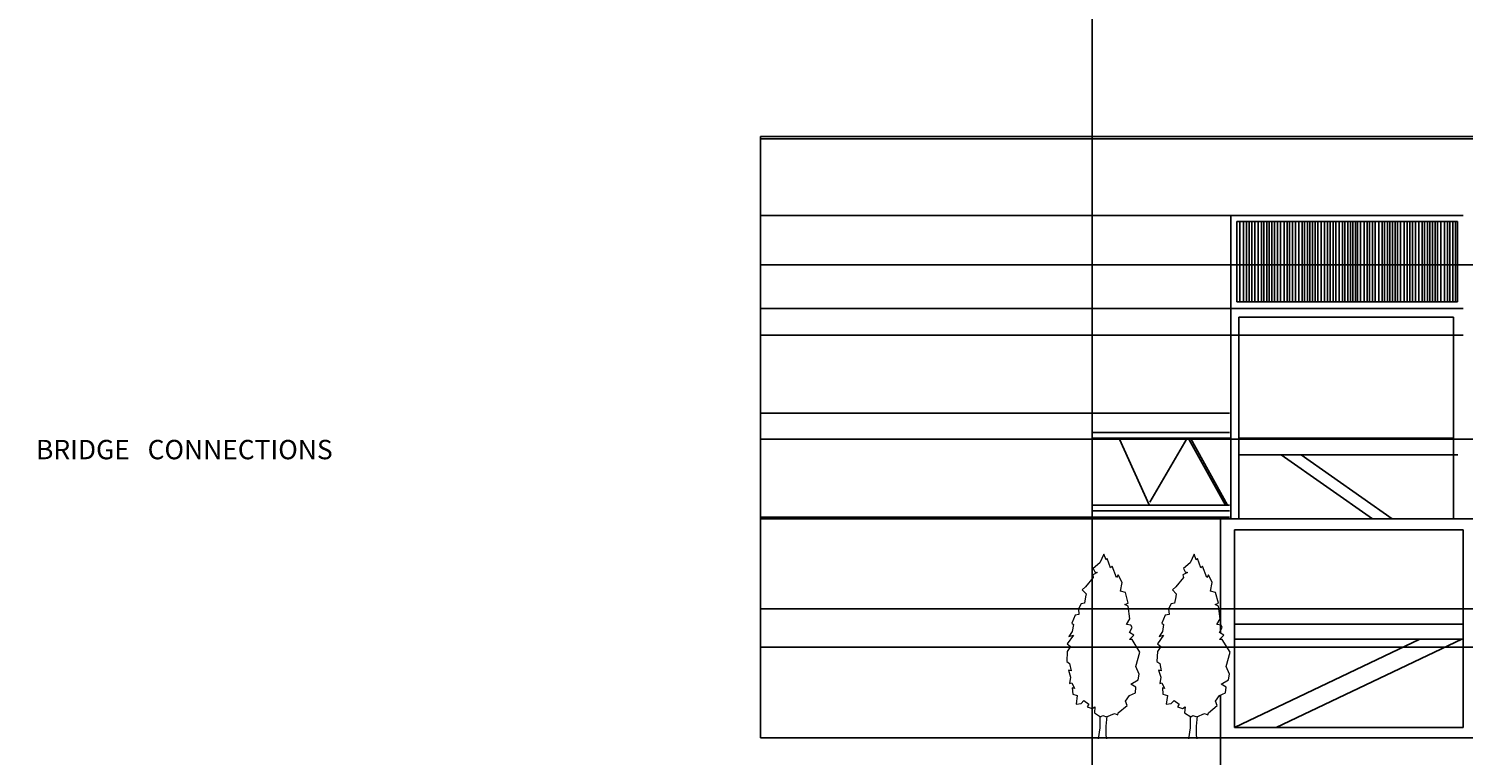
# Model space of a CAD drawing. Units: inches. Extents: x -32109 to 33221, y -19197 to 7608.
# Tile 15 of 25: x -741 to 10957, y -11718 to -5795. Entities that reach past the tile are written whole.
import ezdxf

# ---------------------------------------------------------------- set-up
doc = ezdxf.new("R2010")
doc.units = ezdxf.units.IN
doc.header["$MEASUREMENT"] = 0
for name, color, linetype, lineweight in [('A-ANNO-DIMS', 2, 'Continuous', 18), ('A-ANNO-TEXT', 7, 'Continuous', 25), ('A-ELEV', 7, 'Continuous', 25), ('L-PLNT', 3, 'Continuous', 13)]:
    doc.layers.add(name, color=color, linetype=linetype, lineweight=lineweight)
doc.styles.get("Standard").update_dxf_attribs({"font": 'arial.ttf'})
doc.dimstyles.get("Standard").update_dxf_attribs({"dimtxt": 0.18, "dimasz": 0.18, "dimexe": 0.18, "dimexo": 0.0625, "dimgap": 0.09, "dimtad": 0, "dimtih": 1, "dimtoh": 1, "dimdec": 4, "dimzin": 0, "dimdsep": 46, "dimtxsty": 'Standard', "dimcen": 0.09, "dimadec": 0, "dimazin": 0, "dimtfac": 1, "dimtdec": 4, "dimtofl": 0, "dimtmove": 0, "dimatfit": 3, "dimfxl": 1, "dimtolj": 1, "dimtzin": 0, "dimarcsym": 0})

# ---------------------------------------------------------------- blocks, each defined once
blk = doc.blocks.new('*U2')
blk.add_lwpolyline([(-2.75400000000036, 191.699), (-6.7800000000002, 182.8509999999996), (-13.68200000000024, 176.9529999999995), (-11.95600000000013, 173.2659999999996), (-9.655999999999949, 172.529), (-14.25700000000006, 170.317), (-13.68200000000024, 167.3679999999999), (-21.73300000000017, 157.7829999999999), (-25.1840000000002, 154.8340000000003), (-21.15800000000036, 150.4099999999998), (-21.73300000000017, 147.4609999999998), (-22.88400000000001, 140.8249999999998), (-26.33400000000029, 140.087), (-29.21000000000004, 134.9259999999995), (-28.63499999999977, 129.0279999999998), (-32.66100000000006, 128.2909999999997), (-36.11099999999988, 120.1799999999998), (-34.38599999999997, 118.7059999999997), (-35.53600000000006, 111.3329999999996), (-38.98700000000008, 106.1709999999998), (-34.38599999999997, 107.6459999999997), (-40.71199999999999, 98.79799999999977), (-37.26099999999997, 95.8489999999997), (-40.71199999999999, 90.68799999999965), (-41.28700000000026, 80.36599999999999), (-38.41200000000026, 78.154), (-36.68600000000015, 70.78099999999995), (-39.5619999999999, 71.51799999999957), (-37.26099999999997, 64.14499999999998), (-38.41200000000026, 57.50899999999956), (-36.11099999999988, 58.24699999999984), (-33.23599999999988, 52.3479999999995), (-35.53600000000006, 53.08599999999978), (-34.96100000000024, 46.44999999999981), (-30.36000000000013, 44.9749999999999), (-31.50999999999977, 36.1279999999997), (-26.33400000000029, 36.86499999999978), (-23.45900000000029, 39.81399999999985), (-18.28300000000036, 36.1279999999997), (-20.00800000000027, 33.17799999999988), (-14.83199999999988, 31.70399999999972), (-11.95600000000013, 33.17799999999988), (-12.53099999999995, 27.27999999999975), (-6.204999999999927, 22.85599999999977), (-3.9050000000002, 24.33099999999968), (0.1209999999996398, 22.85599999999977), (8.172999999999774, 26.54299999999967), (11.62399999999979, 25.06799999999976), (12.19900000000007, 27.27999999999975), (21.40000000000009, 34.6529999999998), (19.67500000000018, 39.07699999999977), (23.70099999999957, 44.9749999999999), (30.02700000000004, 47.92399999999997), (30.60199999999986, 53.82299999999986), (25.42599999999993, 56.77199999999993), (32.90299999999979, 61.19599999999991), (34.05299999999988, 67.0939999999996), (30.60199999999986, 75.20499999999993), (34.6279999999997, 89.95100000000002), (26.57599999999957, 103.2219999999997), (23.70099999999957, 103.2219999999997), (28.30199999999968, 107.6459999999997), (23.70099999999957, 110.5949999999998), (26.57599999999957, 115.7559999999994), (25.42599999999993, 117.9679999999998), (20.82499999999982, 118.7059999999997), (24.27599999999984, 124.6040000000002), (22.55099999999993, 137.8759999999997), (19.09999999999991, 139.3499999999999), (22.55099999999993, 140.8249999999998), (19.67500000000018, 151.884), (14.49899999999979, 153.3589999999999), (16.22400000000016, 162.2069999999999), (12.19900000000007, 170.317), (10.47299999999995, 167.3679999999999), (5.871999999999843, 179.1649999999999), (4.146999999999934, 177.69), (0.6959999999999127, 187.2749999999996), (-0.4540000000001783, 185.7999999999997)], close=True)
for points in [[(-6.813000000000101, 23.66899999999987), (-6.813000000000101, 11.66899999999987), (-8.626999999999953, 0)], [(0.3869999999997162, 23.66899999999987), (-0.5760000000000219, 13.27099999999973), (-0.5760000000000219, 3.685999999999694), (0, 0)]]:
    blk.add_lwpolyline(points)
blk = doc.blocks.new('*D14')
at = {"layer": 'A-ANNO-DIMS', "color": 0, "lineweight": -2, "transparency": 16777216}
for p, q in [((-18893.90707200001, -10978.730223), (-32108.36667400003, -10978.73022300001)), ((-32108.18667400003, -10978.91022300001), (-32108.18667400003, -13611.23962386222)), ((-32108.18667400003, -16243.93283100001), (-32108.18667400003, -13611.6034301378)), ((5067.088884000002, -16244.11283100001), (-32108.36667400003, -16244.11283100001))]:
    blk.add_line(p, q, dxfattribs=at)
at = {"layer": 'A-ANNO-DIMS', "color": 0, "transparency": 16777216}
for points in [[(-32108.21667400003, -10978.91022300001), (-32108.15667400003, -10978.91022300001), (-32108.18667400003, -10978.73022300001)], [(-32108.21667400003, -16243.93283100001), (-32108.15667400003, -16243.93283100001), (-32108.18667400003, -16244.11283100001)]]:
    blk.add_solid(points, dxfattribs=at)
at = {"layer": 'Defpoints', "color": 0, "transparency": 16777216}
for p in [(-18893.84457200001, -10978.730223), (-32108.18667400003, -16244.11283100001), (5067.151384000002, -16244.11283100001)]:
    blk.add_point(p, dxfattribs=at)
at = {"layer": 'A-ANNO-DIMS', "color": 0, "transparency": 16777216, "insert": (-32108.18667400002, -13611.421527), "char_height": 0.18, "attachment_point": 5}
blk.add_mtext('\\A1;5265', dxfattribs=at)
blk = doc.blocks.new('*D16')
at = {"layer": 'A-ANNO-DIMS', "color": 0, "lineweight": -2, "transparency": 16777216}
for p, q in [((7931.85712, -8929.002357), (7931.85712, -4467.086268999999)), ((7932.03712, -4467.266268999999), (18774.66361096794, -4467.266268999999)), ((29618.150443, -4467.266268999999), (18775.52395203206, -4467.266268999999)), ((29618.330443, -6090.731526999999), (29618.330443, -4467.086268999999))]:
    blk.add_line(p, q, dxfattribs=at)
at = {"layer": 'A-ANNO-DIMS', "color": 0, "transparency": 16777216}
for points in [[(7932.03712, -4467.236268999999), (7932.03712, -4467.296269), (7931.85712, -4467.266268999999)], [(29618.150443, -4467.236268999999), (29618.150443, -4467.296269), (29618.330443, -4467.266268999999)]]:
    blk.add_solid(points, dxfattribs=at)
at = {"layer": 'Defpoints', "color": 0, "transparency": 16777216}
for p in [(29618.330443, -4467.266268999999), (29618.330443, -6090.794027), (7931.85712, -8929.064857)]:
    blk.add_point(p, dxfattribs=at)
at = {"layer": 'A-ANNO-DIMS', "color": 0, "transparency": 16777216, "insert": (18775.0937815, -4467.266268999999), "char_height": 0.18, "attachment_point": 5}
blk.add_mtext('\\A1;21686', dxfattribs=at)
blk = doc.blocks.new('*D17')
at = {"layer": 'A-ANNO-DIMS', "color": 0, "lineweight": -2, "transparency": 16777216}
for p, q in [((29618.39294300002, -6090.794027000002), (33221.11530000003, -6090.794027000001)), ((33220.93530000003, -6090.974027000001), (33220.93530000003, -8833.116883862214)), ((33220.93530000003, -11575.623547), (33220.93530000003, -8833.48069013779)), ((8978.174905000003, -11575.803547), (33221.11530000003, -11575.803547))]:
    blk.add_line(p, q, dxfattribs=at)
at = {"layer": 'A-ANNO-DIMS', "color": 0, "transparency": 16777216}
for points in [[(33220.90530000003, -6090.974027000001), (33220.96530000003, -6090.974027000001), (33220.93530000003, -6090.794027000001)], [(33220.90530000003, -11575.623547), (33220.96530000003, -11575.623547), (33220.93530000003, -11575.803547)]]:
    blk.add_solid(points, dxfattribs=at)
at = {"layer": 'Defpoints', "color": 0, "transparency": 16777216}
for p in [(29618.33044300001, -6090.794027000002), (8978.112405000002, -11575.803547), (33220.93530000003, -11575.803547)]:
    blk.add_point(p, dxfattribs=at)
at = {"layer": 'A-ANNO-DIMS', "color": 0, "transparency": 16777216, "insert": (33220.93530000002, -8833.298787000009), "char_height": 0.18, "attachment_point": 5}
blk.add_mtext('\\A1;5485', dxfattribs=at)
blk = doc.blocks.new('*D118')
at = {"layer": 'A-ANNO-DIMS', "color": 0, "lineweight": -2, "transparency": 16777216}
for p, q in [((7931.85712, -8929.127357), (7931.85712, -13529.670166)), ((8978.112405, -11575.866047), (8978.112405, -13529.670166)), ((7932.03712, -13529.490166), (8454.529605610505, -13529.490166)), ((8977.932405, -13529.490166), (8455.439919389495, -13529.490166))]:
    blk.add_line(p, q, dxfattribs=at)
at = {"layer": 'A-ANNO-DIMS', "color": 0, "transparency": 16777216}
for points in [[(7932.03712, -13529.460166), (7932.03712, -13529.520166), (7931.85712, -13529.490166)], [(8977.932405, -13529.460166), (8977.932405, -13529.520166), (8978.112405, -13529.490166)]]:
    blk.add_solid(points, dxfattribs=at)
at = {"layer": 'Defpoints', "color": 0, "transparency": 16777216}
for p in [(7931.85712, -8929.064857), (8978.112405, -11575.803547), (8978.112405, -13529.490166)]:
    blk.add_point(p, dxfattribs=at)
at = {"layer": 'A-ANNO-DIMS', "color": 0, "transparency": 16777216, "insert": (8454.9847625, -13529.490166), "char_height": 0.18, "attachment_point": 5}
blk.add_mtext('\\A1;1046.3', dxfattribs=at)
blk = doc.blocks.new('*D119')
at = {"layer": 'A-ANNO-DIMS', "color": 0, "lineweight": -2, "transparency": 16777216}
for p, q in [((8978.112405, -11575.866047), (8978.112405, -13529.670166)), ((11053.824937, -11575.866047), (11053.824937, -13529.670166)), ((8978.292405, -13529.490166), (10015.50350728922, -13529.490166)), ((11053.644937, -13529.490166), (10016.43383471078, -13529.490166))]:
    blk.add_line(p, q, dxfattribs=at)
at = {"layer": 'A-ANNO-DIMS', "color": 0, "transparency": 16777216}
for points in [[(8978.292405, -13529.460166), (8978.292405, -13529.520166), (8978.112405, -13529.490166)], [(11053.644937, -13529.460166), (11053.644937, -13529.520166), (11053.824937, -13529.490166)]]:
    blk.add_solid(points, dxfattribs=at)
at = {"layer": 'Defpoints', "color": 0, "transparency": 16777216}
for p in [(8978.112405, -11575.803547), (11053.824937, -11575.803547), (11053.824937, -13529.490166)]:
    blk.add_point(p, dxfattribs=at)
at = {"layer": 'A-ANNO-DIMS', "color": 0, "transparency": 16777216, "insert": (10015.968671, -13529.490166), "char_height": 0.18, "attachment_point": 5}
blk.add_mtext('\\A1;2075.7', dxfattribs=at)
blk = doc.blocks.new('*D123')
at = {"layer": 'A-ANNO-DIMS', "color": 0, "lineweight": -2, "transparency": 16777216}
for p, q in [((9060.819417000004, -7316.541440000003), (5225.359725000004, -7316.541440000005)), ((5225.539725000004, -7316.721440000005), (5225.539725000004, -9445.990590362215)), ((5225.539725000004, -11575.623547), (5225.539725000004, -9446.354396637793)), ((8978.049905000003, -11575.803547), (5225.359725000004, -11575.803547))]:
    blk.add_line(p, q, dxfattribs=at)
at = {"layer": 'A-ANNO-DIMS', "color": 0, "transparency": 16777216}
for points in [[(5225.509725000003, -7316.721440000005), (5225.569725000003, -7316.721440000005), (5225.539725000004, -7316.541440000005)], [(5225.509725000005, -11575.623547), (5225.569725000004, -11575.623547), (5225.539725000004, -11575.803547)]]:
    blk.add_solid(points, dxfattribs=at)
at = {"layer": 'Defpoints', "color": 0, "transparency": 16777216}
for p in [(9060.881917000004, -7316.541440000003), (5225.539725000004, -11575.803547), (8978.112405000002, -11575.803547)]:
    blk.add_point(p, dxfattribs=at)
at = {"layer": 'A-ANNO-DIMS', "color": 0, "transparency": 16777216, "insert": (5225.539724999999, -9446.172493500004), "char_height": 0.18, "attachment_point": 5}
blk.add_mtext('\\A1;4259', dxfattribs=at)
blk = doc.blocks.new('*D124')
at = {"layer": 'A-ANNO-DIMS', "color": 0, "lineweight": -2, "transparency": 16777216}
for p, q in [((10957.577133, -7316.541440000003), (5225.359725000004, -7316.541440000006)), ((5225.539725000004, -7316.721440000006), (5225.539725000004, -7696.150608362215)), ((5225.539725000004, -8075.943583000004), (5225.539725000004, -7696.514414637795)), ((10957.577133, -8076.123583000002), (5225.359725000004, -8076.123583000004))]:
    blk.add_line(p, q, dxfattribs=at)
at = {"layer": 'A-ANNO-DIMS', "color": 0, "transparency": 16777216}
for points in [[(5225.509725000003, -7316.721440000006), (5225.569725000003, -7316.721440000006), (5225.539725000004, -7316.541440000006)], [(5225.509725000003, -8075.943583000004), (5225.569725000003, -8075.943583000004), (5225.539725000004, -8076.123583000004)]]:
    blk.add_solid(points, dxfattribs=at)
at = {"layer": 'Defpoints', "color": 0, "transparency": 16777216}
for p in [(10957.639633, -7316.541440000003), (5225.539725000004, -8076.123583000004), (10957.639633, -8076.123583000002)]:
    blk.add_point(p, dxfattribs=at)
at = {"layer": 'A-ANNO-DIMS', "color": 0, "transparency": 16777216, "insert": (5225.539724999999, -7696.332511500004), "char_height": 0.18, "attachment_point": 5}
blk.add_mtext('\\A1;759.6', dxfattribs=at)
blk = doc.blocks.new('*D125')
at = {"layer": 'A-ANNO-DIMS', "color": 0, "lineweight": -2, "transparency": 16777216}
for p, q in [((11053.762437, -9789.375425000004), (5225.359725000002, -9789.375425000004)), ((5225.539725000002, -9789.555425000004), (5225.539725000004, -10682.40758286221)), ((5225.539725000004, -11575.623547), (5225.539725000004, -10682.77138913779)), ((11053.762437, -11575.803547), (5225.359725000004, -11575.803547))]:
    blk.add_line(p, q, dxfattribs=at)
at = {"layer": 'A-ANNO-DIMS', "color": 0, "transparency": 16777216}
for points in [[(5225.509725000002, -9789.555425000004), (5225.569725000003, -9789.555425000004), (5225.539725000002, -9789.375425000004)], [(5225.509725000003, -11575.623547), (5225.569725000003, -11575.623547), (5225.539725000004, -11575.803547)]]:
    blk.add_solid(points, dxfattribs=at)
at = {"layer": 'Defpoints', "color": 0, "transparency": 16777216}
for p in [(11053.824937, -9789.375425000004), (5225.539725000004, -11575.803547), (11053.824937, -11575.803547)]:
    blk.add_point(p, dxfattribs=at)
at = {"layer": 'A-ANNO-DIMS', "color": 0, "transparency": 16777216, "insert": (5225.539724999999, -10682.589486), "char_height": 0.18, "attachment_point": 5}
blk.add_mtext('\\A1;1786.4', dxfattribs=at)
blk = doc.blocks.new('*D126')
at = {"layer": 'A-ANNO-DIMS', "color": 0, "lineweight": -2, "transparency": 16777216}
for p, q in [((7931.794620000004, -8929.064857000003), (5225.359725000004, -8929.064857000003)), ((5225.539725000004, -8929.244857000003), (5225.539725000004, -9352.926637862214)), ((5225.539725000004, -9776.972225000003), (5225.539725000004, -9353.290444137792)), ((7931.794620000004, -9777.152225000003), (5225.359725000004, -9777.152225000003))]:
    blk.add_line(p, q, dxfattribs=at)
at = {"layer": 'A-ANNO-DIMS', "color": 0, "transparency": 16777216}
for points in [[(5225.509725000003, -8929.244857000003), (5225.569725000003, -8929.244857000003), (5225.539725000004, -8929.064857000003)], [(5225.509725000003, -9776.972225000003), (5225.569725000003, -9776.972225000003), (5225.539725000004, -9777.152225000003)]]:
    blk.add_solid(points, dxfattribs=at)
at = {"layer": 'Defpoints', "color": 0, "transparency": 16777216}
for p in [(7931.857120000003, -8929.064857000003), (5225.539725000004, -9777.152225000003), (7931.857120000003, -9777.152225000003)]:
    blk.add_point(p, dxfattribs=at)
at = {"layer": 'A-ANNO-DIMS', "color": 0, "transparency": 16777216, "insert": (5225.539724999999, -9353.108541000001), "char_height": 0.18, "attachment_point": 5}
blk.add_mtext('\\A1;848.1', dxfattribs=at)
blk = doc.blocks.new('*D127')
at = {"layer": 'A-ANNO-DIMS', "color": 0, "lineweight": -2, "transparency": 16777216}
for p, q in [((7931.794620000004, -9777.152225000003), (5225.359725000004, -9777.152225000003)), ((5225.539725000002, -9777.332225000004), (5225.539725000004, -10676.29598286221)), ((5225.539725000004, -11575.623547), (5225.539725000004, -10676.65978913779)), ((8978.049905000003, -11575.803547), (5225.359725000004, -11575.803547))]:
    blk.add_line(p, q, dxfattribs=at)
at = {"layer": 'A-ANNO-DIMS', "color": 0, "transparency": 16777216}
for points in [[(5225.509725000002, -9777.332225000004), (5225.569725000003, -9777.332225000004), (5225.539725000002, -9777.152225000003)], [(5225.509725000003, -11575.623547), (5225.569725000003, -11575.623547), (5225.539725000004, -11575.803547)]]:
    blk.add_solid(points, dxfattribs=at)
at = {"layer": 'Defpoints', "color": 0, "transparency": 16777216}
for p in [(7931.857120000003, -9777.152225000003), (5225.539725000004, -11575.803547), (8978.112405000002, -11575.803547)]:
    blk.add_point(p, dxfattribs=at)
at = {"layer": 'A-ANNO-DIMS', "color": 0, "transparency": 16777216, "insert": (5225.539724999999, -10676.477886), "char_height": 0.18, "attachment_point": 5}
blk.add_mtext('\\A1;1798.7', dxfattribs=at)
blk = doc.blocks.new('*D128')
at = {"layer": 'A-ANNO-DIMS', "color": 0, "lineweight": -2, "transparency": 16777216}
for p, q in [((10957.513035, -8293.137571000001), (5225.359725000004, -8293.137571000001)), ((5225.539725000004, -8293.317571000001), (5225.539725000004, -8716.999351862214)), ((5225.539725000004, -9141.044939000003), (5225.539725000004, -8717.36315813779)), ((10957.513035, -9141.224939000003), (5225.359725000004, -9141.224939000003))]:
    blk.add_line(p, q, dxfattribs=at)
at = {"layer": 'A-ANNO-DIMS', "color": 0, "transparency": 16777216}
for points in [[(5225.509725000003, -8293.317571000001), (5225.569725000003, -8293.317571000001), (5225.539725000004, -8293.137571000001)], [(5225.509725000003, -9141.044939000003), (5225.569725000003, -9141.044939000003), (5225.539725000004, -9141.224939000003)]]:
    blk.add_solid(points, dxfattribs=at)
at = {"layer": 'Defpoints', "color": 0, "transparency": 16777216}
for p in [(10957.575535, -8293.137571000001), (5225.539725000004, -9141.224939000003), (10957.575535, -9141.224939000003)]:
    blk.add_point(p, dxfattribs=at)
at = {"layer": 'A-ANNO-DIMS', "color": 0, "transparency": 16777216, "insert": (5225.539724999999, -8717.181255000003), "char_height": 0.18, "attachment_point": 5}
blk.add_mtext('\\A1;848.1', dxfattribs=at)
blk = doc.blocks.new('*D129')
at = {"layer": 'A-ANNO-DIMS', "color": 0, "lineweight": -2, "transparency": 16777216}
for p, q in [((14268.218448, -9141.224939000003), (5225.359725000004, -9141.224939000005)), ((5225.539725000002, -9141.404939000005), (5225.539725000004, -10358.33227847067)), ((5225.539725000004, -11575.623547), (5225.539725000004, -10358.69620752933)), ((12283.489421, -11575.803547), (5225.359725000004, -11575.803547))]:
    blk.add_line(p, q, dxfattribs=at)
at = {"layer": 'A-ANNO-DIMS', "color": 0, "transparency": 16777216}
for points in [[(5225.509725000002, -9141.404939000005), (5225.569725000003, -9141.404939000005), (5225.539725000002, -9141.224939000005)], [(5225.509725000003, -11575.623547), (5225.569725000003, -11575.623547), (5225.539725000004, -11575.803547)]]:
    blk.add_solid(points, dxfattribs=at)
at = {"layer": 'Defpoints', "color": 0, "transparency": 16777216}
for p in [(14268.280948, -9141.224939000003), (5225.539725000004, -11575.803547), (12283.551921, -11575.803547)]:
    blk.add_point(p, dxfattribs=at)
at = {"layer": 'A-ANNO-DIMS', "color": 0, "transparency": 16777216, "insert": (5225.539724999999, -10358.514243), "char_height": 0.18, "attachment_point": 5}
blk.add_mtext('\\A1;2434.6', dxfattribs=at)
blk = doc.blocks.new('*D130')
at = {"layer": 'A-ANNO-DIMS', "color": 0, "lineweight": -2, "transparency": 16777216}
for p, q in [((12283.489421, -10522.894927), (5225.359725000004, -10522.894927)), ((5225.539725000004, -10523.074927), (5225.539725000004, -10680.05586447067)), ((5225.539725000004, -10837.400731), (5225.539725000004, -10680.41979352933)), ((12283.489421, -10837.580731), (5225.359725000004, -10837.580731))]:
    blk.add_line(p, q, dxfattribs=at)
at = {"layer": 'A-ANNO-DIMS', "color": 0, "transparency": 16777216}
for points in [[(5225.509725000003, -10523.074927), (5225.569725000003, -10523.074927), (5225.539725000004, -10522.894927)], [(5225.509725000003, -10837.400731), (5225.569725000003, -10837.400731), (5225.539725000004, -10837.580731)]]:
    blk.add_solid(points, dxfattribs=at)
at = {"layer": 'Defpoints', "color": 0, "transparency": 16777216}
for p in [(12283.551921, -10522.894927), (5225.539725000004, -10837.580731), (12283.551921, -10837.580731)]:
    blk.add_point(p, dxfattribs=at)
at = {"layer": 'A-ANNO-DIMS', "color": 0, "transparency": 16777216, "insert": (5225.539724999999, -10680.237829), "char_height": 0.18, "attachment_point": 5}
blk.add_mtext('\\A1;314.7', dxfattribs=at)
blk = doc.blocks.new('*D131')
at = {"layer": 'A-ANNO-DIMS', "color": 0, "lineweight": -2, "transparency": 16777216}
for p, q in [((16706.62935100001, -6674.260482000004), (5225.359725000004, -6674.260482000005)), ((5225.539725000004, -6674.440482000005), (5225.539725000004, -9124.850111362215)), ((5225.539725000004, -11575.623547), (5225.539725000004, -9125.213917637793)), ((16610.03756200001, -11575.803547), (5225.359725000004, -11575.803547))]:
    blk.add_line(p, q, dxfattribs=at)
at = {"layer": 'A-ANNO-DIMS', "color": 0, "transparency": 16777216}
for points in [[(5225.509725000003, -6674.440482000005), (5225.569725000003, -6674.440482000005), (5225.539725000004, -6674.260482000005)], [(5225.509725000005, -11575.623547), (5225.569725000004, -11575.623547), (5225.539725000004, -11575.803547)]]:
    blk.add_solid(points, dxfattribs=at)
at = {"layer": 'Defpoints', "color": 0, "transparency": 16777216}
for p in [(16706.69185100001, -6674.260482000004), (5225.539725000004, -11575.803547), (16610.10006200001, -11575.803547)]:
    blk.add_point(p, dxfattribs=at)
at = {"layer": 'A-ANNO-DIMS', "color": 0, "transparency": 16777216, "insert": (5225.539724999999, -9125.032014500004), "char_height": 0.18, "attachment_point": 5}
blk.add_mtext('\\A1;4902', dxfattribs=at)
blk = doc.blocks.new('*D132')
at = {"layer": 'A-ANNO-DIMS', "color": 0, "lineweight": -2, "transparency": 16777216}
for p, q in [((16706.62935100001, -6693.379784000004), (5225.359725000004, -6693.379784000005)), ((5225.539725000004, -6693.559784000005), (5225.539725000004, -7206.365229970673)), ((5225.539725000004, -7719.534605000005), (5225.539725000004, -7206.729159029338)), ((16706.62935100001, -7719.714605000004), (5225.359725000004, -7719.714605000006))]:
    blk.add_line(p, q, dxfattribs=at)
at = {"layer": 'A-ANNO-DIMS', "color": 0, "transparency": 16777216}
for points in [[(5225.509725000003, -6693.559784000005), (5225.569725000003, -6693.559784000005), (5225.539725000004, -6693.379784000005)], [(5225.509725000003, -7719.534605000005), (5225.569725000003, -7719.534605000005), (5225.539725000004, -7719.714605000006)]]:
    blk.add_solid(points, dxfattribs=at)
at = {"layer": 'Defpoints', "color": 0, "transparency": 16777216}
for p in [(16706.69185100001, -6693.379784000004), (5225.539725000004, -7719.714605000006), (16706.69185100001, -7719.714605000004)]:
    blk.add_point(p, dxfattribs=at)
at = {"layer": 'A-ANNO-DIMS', "color": 0, "transparency": 16777216, "insert": (5225.539725, -7206.547194500004), "char_height": 0.18, "attachment_point": 5}
blk.add_mtext('\\A1;1026.3', dxfattribs=at)
blk = doc.blocks.new('*D133')
at = {"layer": 'A-ANNO-DIMS', "color": 0, "lineweight": -2, "transparency": 16777216}
for p, q in [((16706.62935100001, -7719.714605000004), (5225.359725000004, -7719.714605000006)), ((5225.539725000004, -7719.894605000006), (5225.539725000004, -9647.577111470673)), ((5225.539725000004, -11575.623547), (5225.539725000004, -9647.941040529337)), ((16610.03756200001, -11575.803547), (5225.359725000004, -11575.803547))]:
    blk.add_line(p, q, dxfattribs=at)
at = {"layer": 'A-ANNO-DIMS', "color": 0, "transparency": 16777216}
for points in [[(5225.509725000003, -7719.894605000006), (5225.569725000003, -7719.894605000006), (5225.539725000004, -7719.714605000006)], [(5225.509725000005, -11575.623547), (5225.569725000004, -11575.623547), (5225.539725000004, -11575.803547)]]:
    blk.add_solid(points, dxfattribs=at)
at = {"layer": 'Defpoints', "color": 0, "transparency": 16777216}
for p in [(16706.69185100001, -7719.714605000004), (5225.539725000004, -11575.803547), (16610.10006200001, -11575.803547)]:
    blk.add_point(p, dxfattribs=at)
at = {"layer": 'A-ANNO-DIMS', "color": 0, "transparency": 16777216, "insert": (5225.539724999999, -9647.759076000006), "char_height": 0.18, "attachment_point": 5}
blk.add_mtext('\\A1;3856', dxfattribs=at)

msp = doc.modelspace()

# ---------------------------------------------------------------- linework, layer by layer
at = {"layer": 'A-ELEV'}
for p, q in [((9060.88191700589, -7316.541440451536), (9060.88191700589, -8076.123582546014)), ((10957.63963269253, -7316.541440451536), (9060.88191700589, -7316.541440451536)), ((9110.485568459386, -7366.206414277622), (9110.485568459386, -8021.954421354015)), ((9110.485568459386, -7366.206414277622), (10909.67896176421, -7366.206414277622)), ((9136.514483598005, -8021.954421354015), (9136.514483598005, -7366.206414277622)), ((9165.840668374381, -8021.954421354015), (9165.840668374381, -7366.206414277622)), ((9190.14321119021, -8021.954421354015), (9190.14321119021, -7366.206414277622)), ((9210.027139092948, -8021.954421354015), (9210.027139092948, -7366.206414277622)), ((9234.329722107235, -8021.954421354015), (9234.329722107235, -7366.206414277622)), ((9256.42299766499, -8021.954421354015), (9256.42299766499, -7366.206414277622)), ((9285.144195592366, -8021.954421354015), (9285.144195592366, -7366.206414277622)), ((9311.656126261652, -8021.954421354015), (9311.656126261652, -7366.206414277622)), ((9331.540054164398, -8021.954421354015), (9331.540054164398, -7366.206414277622)), ((9355.842596980227, -8021.954421354015), (9355.842596980227, -7366.206414277622)), ((9375.726524882963, -8021.954421354015), (9375.726524882963, -7366.206414277622)), ((9395.610452785708, -8021.954421354015), (9395.610452785708, -7366.206414277622)), ((9417.703728343447, -8021.954421354015), (9417.703728343447, -7366.206414277622)), ((9441.884340039425, -7366.206414277622), (9441.884340039425, -8021.954421354015)), ((9467.913255178037, -8021.954421354015), (9467.913255178037, -7366.206414277622)), ((9497.239439954406, -8021.954421354015), (9497.239439954406, -7366.206414277622)), ((9521.541982770243, -8021.954421354015), (9521.541982770243, -7366.206414277622)), ((9541.42591067298, -8021.954421354015), (9541.42591067298, -7366.206414277622)), ((9565.728493687267, -8021.954421354015), (9565.728493687267, -7366.206414277622)), ((9587.821769245022, -8021.954421354015), (9587.821769245022, -7366.206414277622)), ((9616.5429671724, -8021.954421354015), (9616.5429671724, -7366.206414277622)), ((9643.054897841686, -8021.954421354015), (9643.054897841686, -7366.206414277622)), ((9662.938825744432, -8021.954421354015), (9662.938825744432, -7366.206414277622)), ((9687.24136856025, -8021.954421354015), (9687.24136856025, -7366.206414277622)), ((9707.125296462997, -8021.954421354015), (9707.125296462997, -7366.206414277622)), ((9727.009224365735, -8021.954421354015), (9727.009224365735, -7366.206414277622)), ((9749.10249992348, -8021.954421354015), (9749.10249992348, -7366.206414277622)), ((9771.073804162917, -7366.206414277622), (9771.073804162917, -8021.954421354015)), ((9797.102719301527, -8021.954421354015), (9797.102719301527, -7366.206414277622)), ((9826.428904077899, -8021.954421354015), (9826.428904077899, -7366.206414277622)), ((9850.731446893726, -8021.954421354015), (9850.731446893726, -7366.206414277622)), ((9870.61537479647, -8021.954421354015), (9870.61537479647, -7366.206414277622)), ((9894.917957810758, -8021.954421354015), (9894.917957810758, -7366.206414277622)), ((9917.01123336851, -8021.954421354015), (9917.01123336851, -7366.206414277622)), ((9945.732431295888, -8021.954421354015), (9945.732431295888, -7366.206414277622)), ((9972.244361965175, -8021.954421354015), (9972.244361965175, -7366.206414277622)), ((9992.12828986792, -8021.954421354015), (9992.12828986792, -7366.206414277622)), ((10016.43083268374, -8021.954421354015), (10016.43083268374, -7366.206414277622)), ((10036.31476058648, -8021.954421354015), (10036.31476058648, -7366.206414277622)), ((10056.19868848922, -8021.954421354015), (10056.19868848922, -7366.206414277622)), ((10078.29196404697, -8021.954421354015), (10078.29196404697, -7366.206414277622)), ((10093.63526551984, -7366.206414277622), (10093.63526551984, -8021.954421354015)), ((10119.66418065846, -8021.954421354015), (10119.66418065846, -7366.206414277622)), ((10148.99036543484, -8021.954421354015), (10148.99036543484, -7366.206414277622)), ((10173.29290825067, -8021.954421354015), (10173.29290825067, -7366.206414277622)), ((10193.1768361534, -8021.954421354015), (10193.1768361534, -7366.206414277622)), ((10217.47941916769, -8021.954421354015), (10217.47941916769, -7366.206414277622)), ((10239.57269472544, -8021.954421354015), (10239.57269472544, -7366.206414277622)), ((10268.29389265281, -8021.954421354015), (10268.29389265281, -7366.206414277622)), ((10294.80582332211, -8021.954421354015), (10294.80582332211, -7366.206414277622)), ((10314.68975122485, -8021.954421354015), (10314.68975122485, -7366.206414277622)), ((10338.99229404067, -8021.954421354015), (10338.99229404067, -7366.206414277622)), ((10358.87622194342, -8021.954421354015), (10358.87622194342, -7366.206414277622)), ((10378.76014984616, -8021.954421354015), (10378.76014984616, -7366.206414277622)), ((10400.8534254039, -8021.954421354015), (10400.8534254039, -7366.206414277622)), ((10420.61538198832, -7366.206414277622), (10420.61538198832, -8021.954421354015)), ((10446.64429712693, -8021.954421354015), (10446.64429712693, -7366.206414277622)), ((10475.97048190331, -8021.954421354015), (10475.97048190331, -7366.206414277622)), ((10500.27302471914, -8021.954421354015), (10500.27302471914, -7366.206414277622)), ((10520.15695262188, -8021.954421354015), (10520.15695262188, -7366.206414277622)), ((10544.45953563617, -8021.954421354015), (10544.45953563617, -7366.206414277622)), ((10566.55281119392, -8021.954421354015), (10566.55281119392, -7366.206414277622)), ((10595.2740091213, -8021.954421354015), (10595.2740091213, -7366.206414277622)), ((10621.78593979059, -8021.954421354015), (10621.78593979059, -7366.206414277622)), ((10641.66986769333, -8021.954421354015), (10641.66986769333, -7366.206414277622)), ((10665.97241050916, -8021.954421354015), (10665.97241050916, -7366.206414277622)), ((10685.8563384119, -8021.954421354015), (10685.8563384119, -7366.206414277622)), ((10705.74026631463, -8021.954421354015), (10705.74026631463, -7366.206414277622)), ((10727.83354187238, -8021.954421354015), (10727.83354187238, -7366.206414277622)), ((10747.59553865527, -7366.206414277622), (10747.59553865527, -8021.954421354015)), ((10773.62445379388, -8021.954421354015), (10773.62445379388, -7366.206414277622)), ((10802.95063857026, -8021.954421354015), (10802.95063857026, -7366.206414277622)), ((10827.2531813861, -8021.954421354015), (10827.2531813861, -7366.206414277622)), ((10847.13710928883, -8021.954421354015), (10847.13710928883, -7366.206414277622)), ((10871.43969230312, -8021.954421354015), (10871.43969230312, -7366.206414277622)), ((10893.53296786087, -8021.954421354015), (10893.53296786087, -7366.206414277622)), ((10909.67896176421, -8021.954421354015), (10909.67896176421, -7366.206414277622)), ((9110.485568459386, -8021.954421354015), (10909.67896176421, -8021.954421354015)), ((9060.88191700589, -8076.123582546014), (10957.63963269253, -8076.123582546014)), ((9060.88191700589, -8076.123582546014), (9060.88191700589, -9789.37542525009)), ((9127.601312008097, -8147.271051415478), (10877.59424882554, -8147.271051415478)), ((9127.601312008097, -9789.37542525009), (9127.601312008097, -8147.271051415478)), ((10877.59424882554, -8147.271051415478), (10877.59424882554, -9789.37542525009)), ((9051.81488447349, -8929.064857346351), (7931.8571203095, -8929.064857346351)), ((7931.8571203095, -8929.064857346351), (7931.8571203095, -9777.15222528266)), ((9051.81488447349, -9086.192961227614), (7931.8571203095, -9086.192961227614)), ((9051.81488447349, -9133.163383348518), (7931.8571203095, -9133.163383348518)), ((8396.727008144362, -9677.277923033176), (8154.646439816509, -9139.867987711146)), ((8706.117419952277, -9133.163383348518), (8402.565919928928, -9655.291652604763)), ((9019.116486171055, -9678.007332945996), (8718.891556173561, -9139.749653560115)), ((9035.552045459453, -9678.007332945996), (8731.653479972952, -9133.163383348518)), ((9051.814884473513, -9133.163383348521), (9060.88191700589, -9133.163383348521)), ((9127.601312008097, -9133.163383348525), (10877.59424882554, -9133.163383348521)), ((9127.601312008097, -9268.825304176527), (10911.54964827016, -9268.825304176524)), ((9473.241069009871, -9268.82530417652), (10216.06358682015, -9789.375425250091)), ((9635.868099057234, -9268.82530417652), (10378.69061686752, -9789.375425250091)), ((9051.81488447349, -9678.007332945996), (7931.8571203095, -9678.007332945996)), ((7931.8571203095, -9724.286537259415), (9051.81488447349, -9724.286537259415)), ((9051.81488447349, -9777.152225282654), (7931.8571203095, -9777.152225282654)), ((8978.112404962298, -9789.37542525009), (11053.82493697622, -9789.37542525009)), ((8978.112404962298, -10721.07407709044), (8978.112404962298, -9789.37542525009)), ((9091.935876885284, -11489.80296378181), (9091.935876885284, -9880.070497759041)), ((9091.935876885284, -9880.070497759041), (9127.601312008097, -9880.070497759041)), ((9127.601312008097, -9880.070497759041), (9127.601312008097, -9880.070497759041)), ((9127.601312008097, -9880.070497759041), (10957.33057972089, -9880.070497759041)), ((10957.33057972089, -9880.070497759041), (10957.33057972089, -11489.80296378181)), ((9091.935876885284, -10648.05454661561), (10957.33057972089, -10648.05454661561)), ((8978.112404962298, -10773.54131612916), (8978.112404962298, -10765.33933916773)), ((9091.935876885284, -10772.4110213961), (10957.33057972089, -10772.4110213961)), ((9091.935876885269, -11489.80296378181), (10604.14114306648, -10772.4110213961)), ((9432.216789609078, -11489.80296378181), (10944.4220557903, -10772.4110213961)), ((8978.112404962298, -11575.80354668384), (8978.112404962298, -11227.25055600641)), ((7931.857120309491, -11575.80354668384), (6605.539725432871, -11575.80354668384)), ((6605.539725432871, -11575.80354668384), (6605.539725432871, -11575.80354668384)), ((6605.539725432871, -11575.80354668384), (31840.93529984972, -11575.80354668384)), ((8978.112404962294, -11575.80354668384), (7931.8571203095, -11575.80354668384)), ((11053.82493697622, -11575.80354668384), (8978.112404962298, -11575.80354668384)), ((10957.33057972089, -11489.80296378181), (9091.935876885284, -11489.80296378181))]:
    msp.add_line(p, q, dxfattribs=at)

# ---------------------------------------------------------------- block references
at = {"layer": 'L-PLNT', "xscale": 7.857670648127824, "yscale": 7.857670648127824, "zscale": 7.857670648127824}
for p in [(8047.947999309682, -11584.62579577021), (8783.347622732215, -11584.62579577021)]:
    msp.add_blockref('*U2', p, dxfattribs=at)

# ---------------------------------------------------------------- texts
at = {"layer": 'A-ANNO-TEXT'}
msp.add_text('SKY   BRIDGE   CONNECTIONS', height=157.8985042017455, dxfattribs=at).set_placement((-1207.497713132039, -9304.611995487214))

# ---------------------------------------------------------------- dimensions: what is measured, and where the dimension line sits
at = {"layer": 'A-ANNO-DIMS'}
for base, p1, p2, override, picture, middle in [((29618.330443, -4467.266268999999), (7931.85712, -8929.064857), (29618.330443, -6090.794027), {"dimdec": 0, "dimlfac": 1, "dimrnd": 0, "dimzin": 0, "dimdsep": 46, "dimlunit": 2}, '*D16', (18775.0937815, -4467.266268999999)), ((8978.112405, -13529.490166), (7931.85712, -8929.064857), (8978.112405, -11575.803547), {"dimdec": 1, "dimlfac": 1, "dimrnd": 0, "dimzin": 0, "dimdsep": 46, "dimlunit": 2}, '*D118', (8454.9847625, -13529.490166)), ((11053.824937, -13529.490166), (8978.112405, -11575.803547), (11053.824937, -11575.803547), {"dimdec": 1, "dimlfac": 1, "dimrnd": 0, "dimzin": 0, "dimdsep": 46, "dimlunit": 2}, '*D119', (10015.968671, -13529.490166))]:
    dim = msp.add_linear_dim(base=base, p1=p1, p2=p2, dimstyle='Standard', override=override, dxfattribs=at)
    dim.commit()
    dim.dimension.update_dxf_attribs({"geometry": picture, "text_midpoint": middle})
for base, p1, p2, override, picture, middle in [((33220.93530000003, -11575.803547), (29618.330443, -6090.794027), (8978.112405, -11575.803547), {"dimdec": 0, "dimlfac": 1, "dimrnd": 0, "dimzin": 0, "dimdsep": 46, "dimlunit": 2}, '*D17', (33220.93530000002, -8833.298787000009)), ((5225.539725000004, -7719.714605000006), (16706.691851, -6693.379784), (16706.691851, -7719.714605), {"dimdec": 1, "dimlfac": 1, "dimrnd": 0, "dimzin": 0, "dimdsep": 46, "dimlunit": 2}, '*D132', (5225.539725, -7206.547194500004)), ((5225.539725000004, -11575.803547), (16706.691851, -6674.260482), (16610.100062, -11575.803547), {"dimdec": 0, "dimlfac": 1, "dimrnd": 0, "dimzin": 0, "dimdsep": 46, "dimlunit": 2}, '*D131', (5225.539724999999, -9125.032014500004)), ((5225.539725000004, -8076.123583000004), (10957.639633, -7316.54144), (10957.639633, -8076.123583000001), {"dimdec": 1, "dimlfac": 1, "dimrnd": 0, "dimzin": 0, "dimdsep": 46, "dimlunit": 2}, '*D124', (5225.539724999999, -7696.332511500004)), ((5225.539725000004, -11575.803547), (9060.881917, -7316.54144), (8978.112405, -11575.803547), {"dimdec": 0, "dimlfac": 1, "dimrnd": 0, "dimzin": 0, "dimdsep": 46, "dimlunit": 2}, '*D123', (5225.539724999999, -9446.172493500004)), ((5225.539725000004, -11575.803547), (16706.691851, -7719.714605), (16610.100062, -11575.803547), {"dimdec": 0, "dimlfac": 1, "dimrnd": 0, "dimzin": 0, "dimdsep": 46, "dimlunit": 2}, '*D133', (5225.539724999999, -9647.759076000006)), ((5225.539725000004, -9141.224939000003), (10957.575535, -8293.137571), (10957.575535, -9141.224939), {"dimdec": 1, "dimlfac": 1, "dimrnd": 0, "dimzin": 0, "dimdsep": 46, "dimlunit": 2}, '*D128', (5225.539724999999, -8717.181255000003)), ((5225.539725000004, -9777.152225000003), (7931.85712, -8929.064857), (7931.85712, -9777.152225000002), {"dimdec": 1, "dimlfac": 1, "dimrnd": 0, "dimzin": 0, "dimdsep": 46, "dimlunit": 2}, '*D126', (5225.539724999999, -9353.108541000001)), ((5225.539725000004, -11575.803547), (14268.280948, -9141.224939), (12283.551921, -11575.803547), {"dimdec": 1, "dimlfac": 1, "dimrnd": 0, "dimzin": 0, "dimdsep": 46, "dimlunit": 2}, '*D129', (5225.539724999999, -10358.514243)), ((5225.539725000004, -11575.803547), (7931.85712, -9777.152225000002), (8978.112405, -11575.803547), {"dimdec": 1, "dimlfac": 1, "dimrnd": 0, "dimzin": 0, "dimdsep": 46, "dimlunit": 2}, '*D127', (5225.539724999999, -10676.477886)), ((5225.539725000004, -11575.803547), (11053.824937, -9789.375425), (11053.824937, -11575.803547), {"dimdec": 1, "dimlfac": 1, "dimrnd": 0, "dimzin": 0, "dimdsep": 46, "dimlunit": 2}, '*D125', (5225.539724999999, -10682.589486)), ((5225.539725000004, -10837.580731), (12283.551921, -10522.894927), (12283.551921, -10837.580731), {"dimdec": 1, "dimlfac": 1, "dimrnd": 0, "dimzin": 0, "dimdsep": 46, "dimlunit": 2}, '*D130', (5225.539724999999, -10680.237829)), ((-32108.18667400003, -16244.11283100001), (-18893.844572, -10978.730223), (5067.151383999999, -16244.112831), {"dimdec": 0, "dimlfac": 1, "dimrnd": 0, "dimzin": 0, "dimdsep": 46, "dimlunit": 2}, '*D14', (-32108.18667400002, -13611.421527))]:
    dim = msp.add_linear_dim(base=base, p1=p1, p2=p2, angle=90, dimstyle='Standard', override=override, dxfattribs=at)
    dim.commit()
    dim.dimension.update_dxf_attribs({"geometry": picture, "text_midpoint": middle})

doc.saveas('drawing.dxf')
